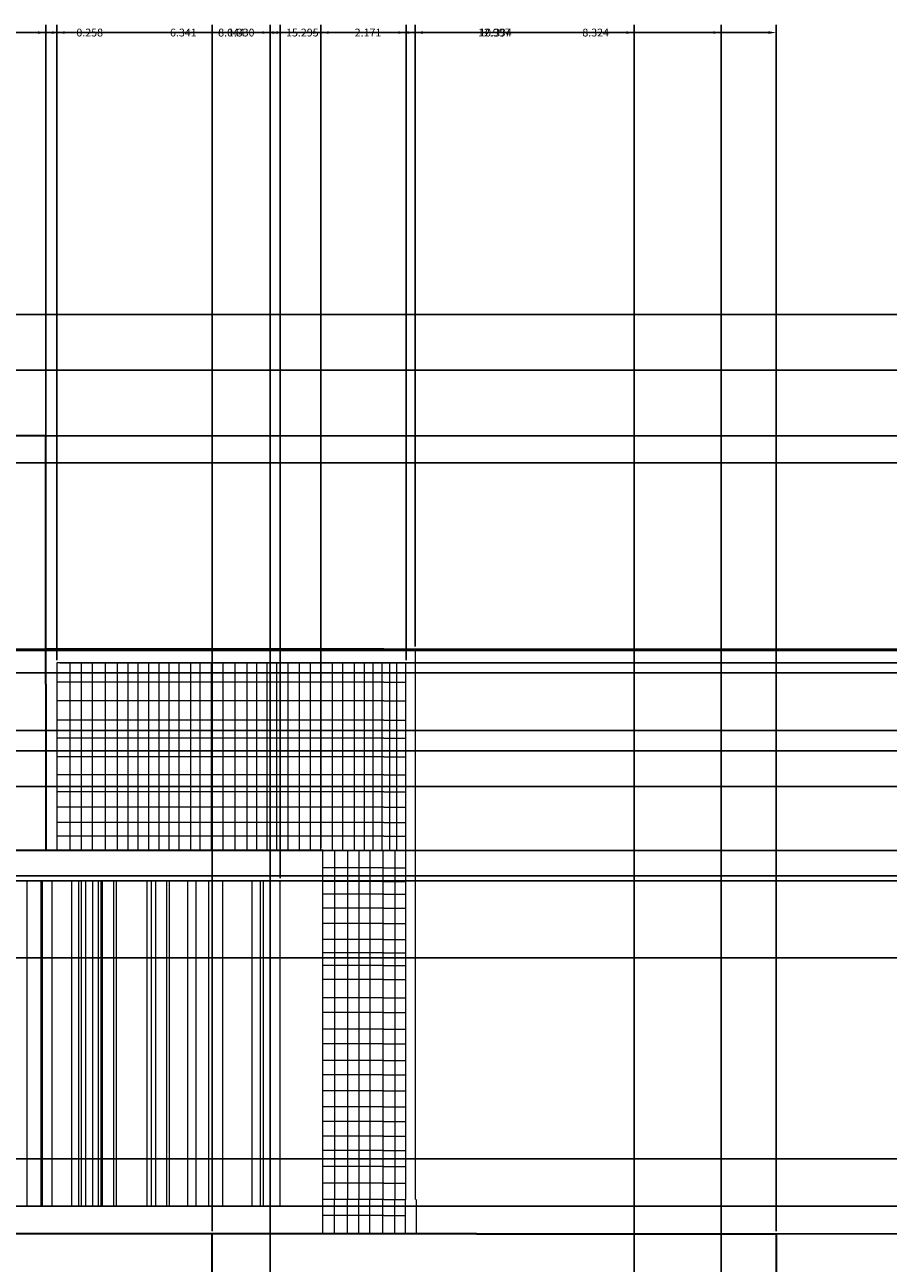
# Model space of a CAD drawing. Units: inches. Extents: x -10 to 130, y -32 to 34.
# Tile 21 of 22: x 90 to 110, y 5 to 34. Entities that reach past the tile are written whole.
import ezdxf

# ---------------------------------------------------------------- set-up
doc = ezdxf.new("R2010")
doc.units = ezdxf.units.IN
doc.header["$MEASUREMENT"] = 0
for name, color, linetype, lineweight in [('A-ANNO-DIMS', 2, 'Continuous', 18), ('A-ELEV', 7, 'Continuous', 35), ('A-GLAZ', 4, 'Continuous', 18)]:
    doc.layers.add(name, color=color, linetype=linetype, lineweight=lineweight)
doc.styles.get("Standard").update_dxf_attribs({"font": 'arial.ttf'})
doc.dimstyles.get("Standard").update_dxf_attribs({"dimtxt": 0.18, "dimasz": 0.18, "dimexe": 0.18, "dimexo": 0.0625, "dimgap": 0.09, "dimtad": 0, "dimtih": 1, "dimtoh": 1, "dimdec": 4, "dimzin": 0, "dimdsep": 46, "dimtxsty": 'Standard', "dimcen": 0.09, "dimadec": 0, "dimazin": 0, "dimtfac": 1, "dimtdec": 4, "dimtofl": 0, "dimtmove": 0, "dimatfit": 3, "dimfxl": 1, "dimtolj": 1, "dimtzin": 0, "dimarcsym": 0})

# ---------------------------------------------------------------- blocks, each defined once
blk = doc.blocks.new('*D2')
at = {"layer": 'A-ANNO-DIMS', "color": 0, "lineweight": -2, "transparency": 16777216}
for p, q in [((68.738, 27.199), (129.508, 27.199)), ((129.328, 27.019), (129.328, 3.074)), ((129.328, -21.234), (129.328, 2.71)), ((107.996, -21.414), (129.508, -21.414))]:
    blk.add_line(p, q, dxfattribs=at)
at = {"layer": 'A-ANNO-DIMS', "color": 0, "transparency": 16777216}
for points in [[(129.298, 27.019), (129.358, 27.019), (129.328, 27.199)], [(129.298, -21.234), (129.358, -21.234), (129.328, -21.414)]]:
    blk.add_solid(points, dxfattribs=at)
at = {"layer": 'Defpoints', "color": 0, "transparency": 16777216}
for p in [(68.676, 27.199), (129.328, 27.199), (107.933, -21.414)]:
    blk.add_point(p, dxfattribs=at)
at = {"layer": 'A-ANNO-DIMS', "color": 0, "transparency": 16777216, "insert": (129.328, 2.892), "char_height": 0.18, "attachment_point": 5}
blk.add_mtext('\\A1;48.61', dxfattribs=at)
blk = doc.blocks.new('*D10')
at = {"layer": 'A-ANNO-DIMS', "color": 0, "lineweight": -2, "transparency": 16777216}
for p, q in [((94.73, 6.07), (94.73, 33.879)), ((94.91, 33.699), (100.773, 33.699)), ((107.547, 33.699), (101.684, 33.699)), ((107.727, 6.07), (107.727, 33.879))]:
    blk.add_line(p, q, dxfattribs=at)
at = {"layer": 'A-ANNO-DIMS', "color": 0, "transparency": 16777216}
for points in [[(94.91, 33.729), (94.91, 33.669), (94.73, 33.699)], [(107.547, 33.729), (107.547, 33.669), (107.727, 33.699)]]:
    blk.add_solid(points, dxfattribs=at)
at = {"layer": 'Defpoints', "color": 0, "transparency": 16777216}
for p in [(107.727, 33.699), (94.73, 6.007), (107.727, 6.007)]:
    blk.add_point(p, dxfattribs=at)
at = {"layer": 'A-ANNO-DIMS', "color": 0, "transparency": 16777216, "insert": (101.229, 33.699), "char_height": 0.18, "attachment_point": 5}
blk.add_mtext('\\A1;12.997', dxfattribs=at)
blk = doc.blocks.new('*D24')
at = {"layer": 'A-ANNO-DIMS', "color": 0, "lineweight": -2, "transparency": 16777216}
for p, q in [((85.383, 19.52), (85.383, 33.879)), ((85.563, 33.699), (87.744, 33.699)), ((90.712, 33.699), (88.531, 33.699)), ((90.892, 24.464), (90.892, 33.879))]:
    blk.add_line(p, q, dxfattribs=at)
at = {"layer": 'A-ANNO-DIMS', "color": 0, "transparency": 16777216}
for points in [[(85.563, 33.729), (85.563, 33.669), (85.383, 33.699)], [(90.712, 33.729), (90.712, 33.669), (90.892, 33.699)]]:
    blk.add_solid(points, dxfattribs=at)
at = {"layer": 'Defpoints', "color": 0, "transparency": 16777216}
for p in [(90.892, 33.699), (90.892, 24.402), (85.383, 19.458)]:
    blk.add_point(p, dxfattribs=at)
at = {"layer": 'A-ANNO-DIMS', "color": 0, "transparency": 16777216, "insert": (88.138, 33.699), "char_height": 0.18, "attachment_point": 5}
blk.add_mtext('\\A1;5.508', dxfattribs=at)
blk = doc.blocks.new('*D25')
at = {"layer": 'A-ANNO-DIMS', "color": 0, "lineweight": -2, "transparency": 16777216}
for p, q in [((90.892, 24.464), (90.892, 33.879)), ((91.072, 33.699), (93.685, 33.699)), ((97.053, 33.699), (94.439, 33.699)), ((97.233, 14.903), (97.233, 33.879))]:
    blk.add_line(p, q, dxfattribs=at)
at = {"layer": 'A-ANNO-DIMS', "color": 0, "transparency": 16777216}
for points in [[(91.072, 33.729), (91.072, 33.669), (90.892, 33.699)], [(97.053, 33.729), (97.053, 33.669), (97.233, 33.699)]]:
    blk.add_solid(points, dxfattribs=at)
at = {"layer": 'Defpoints', "color": 0, "transparency": 16777216}
for p in [(97.233, 33.699), (90.892, 24.402), (97.233, 14.841)]:
    blk.add_point(p, dxfattribs=at)
at = {"layer": 'A-ANNO-DIMS', "color": 0, "transparency": 16777216, "insert": (94.062, 33.699), "char_height": 0.18, "attachment_point": 5}
blk.add_mtext('\\A1;6.341', dxfattribs=at)
blk = doc.blocks.new('*D26')
at = {"layer": 'A-ANNO-DIMS', "color": 0, "lineweight": -2, "transparency": 16777216}
for p, q in [((97.233, 14.903), (97.233, 33.879)), ((97.413, 33.699), (97.94, 33.699)), ((99.223, 33.699), (98.696, 33.699)), ((99.403, 19.547), (99.403, 33.879))]:
    blk.add_line(p, q, dxfattribs=at)
at = {"layer": 'A-ANNO-DIMS', "color": 0, "transparency": 16777216}
for points in [[(97.413, 33.729), (97.413, 33.669), (97.233, 33.699)], [(99.223, 33.729), (99.223, 33.669), (99.403, 33.699)]]:
    blk.add_solid(points, dxfattribs=at)
at = {"layer": 'Defpoints', "color": 0, "transparency": 16777216}
for p in [(99.403, 33.699), (99.403, 19.485), (97.233, 14.841)]:
    blk.add_point(p, dxfattribs=at)
at = {"layer": 'A-ANNO-DIMS', "color": 0, "transparency": 16777216, "insert": (98.318, 33.699), "char_height": 0.18, "attachment_point": 5}
blk.add_mtext('\\A1;2.171', dxfattribs=at)
blk = doc.blocks.new('*D27')
at = {"layer": 'A-ANNO-DIMS', "color": 0, "lineweight": -2, "transparency": 16777216}
for p, q in [((99.403, 19.547), (99.403, 33.879)), ((99.583, 33.699), (103.172, 33.699)), ((107.547, 33.699), (103.959, 33.699)), ((107.727, 6.07), (107.727, 33.879))]:
    blk.add_line(p, q, dxfattribs=at)
at = {"layer": 'A-ANNO-DIMS', "color": 0, "transparency": 16777216}
for points in [[(99.583, 33.729), (99.583, 33.669), (99.403, 33.699)], [(107.547, 33.729), (107.547, 33.669), (107.727, 33.699)]]:
    blk.add_solid(points, dxfattribs=at)
at = {"layer": 'Defpoints', "color": 0, "transparency": 16777216}
for p in [(107.727, 33.699), (99.403, 19.485), (107.727, 6.007)]:
    blk.add_point(p, dxfattribs=at)
at = {"layer": 'A-ANNO-DIMS', "color": 0, "transparency": 16777216, "insert": (103.565, 33.699), "char_height": 0.18, "attachment_point": 5}
blk.add_mtext('\\A1;8.324', dxfattribs=at)
blk = doc.blocks.new('*D29')
at = {"layer": 'A-ANNO-DIMS', "color": 0, "lineweight": -2, "transparency": 16777216}
for p, q in [((69.045, 14.903), (69.045, 33.879)), ((69.225, 33.699), (82.743, 33.699)), ((97.053, 33.699), (83.534, 33.699)), ((97.233, 14.903), (97.233, 33.879))]:
    blk.add_line(p, q, dxfattribs=at)
at = {"layer": 'A-ANNO-DIMS', "color": 0, "transparency": 16777216}
for points in [[(69.225, 33.729), (69.225, 33.669), (69.045, 33.699)], [(97.053, 33.729), (97.053, 33.669), (97.233, 33.699)]]:
    blk.add_solid(points, dxfattribs=at)
at = {"layer": 'Defpoints', "color": 0, "transparency": 16777216}
for p in [(97.233, 33.699), (69.045, 14.841), (97.233, 14.841)]:
    blk.add_point(p, dxfattribs=at)
at = {"layer": 'A-ANNO-DIMS', "color": 0, "transparency": 16777216, "insert": (83.139, 33.699), "char_height": 0.18, "attachment_point": 5}
blk.add_mtext('\\A1;28.19', dxfattribs=at)
blk = doc.blocks.new('*D66')
at = {"layer": 'A-ANNO-DIMS', "color": 0, "lineweight": -2, "transparency": 16777216}
for p, q in [((89.158, -16.844), (89.158, 33.879)), ((89.338, 33.699), (96.35, 33.699)), ((104.273, 33.699), (97.261, 33.699)), ((104.453, -13.219), (104.453, 33.879))]:
    blk.add_line(p, q, dxfattribs=at)
at = {"layer": 'A-ANNO-DIMS', "color": 0, "transparency": 16777216}
for points in [[(89.338, 33.729), (89.338, 33.669), (89.158, 33.699)], [(104.273, 33.729), (104.273, 33.669), (104.453, 33.699)]]:
    blk.add_solid(points, dxfattribs=at)
at = {"layer": 'Defpoints', "color": 0, "transparency": 16777216}
for p in [(104.453, 33.699), (104.453, -13.282), (89.158, -16.906)]:
    blk.add_point(p, dxfattribs=at)
at = {"layer": 'A-ANNO-DIMS', "color": 0, "transparency": 16777216, "insert": (96.805, 33.699), "char_height": 0.18, "attachment_point": 5}
blk.add_mtext('\\A1;15.295', dxfattribs=at)
blk = doc.blocks.new('*D79')
at = {"layer": 'A-ANNO-DIMS', "color": 0, "lineweight": -2, "transparency": 16777216}
for p, q in [((62.588, 7.736), (129.508, 7.736)), ((129.328, 7.556), (129.328, 5.559)), ((129.328, 3.198), (129.328, 5.195)), ((62.588, 3.018), (129.508, 3.018))]:
    blk.add_line(p, q, dxfattribs=at)
at = {"layer": 'A-ANNO-DIMS', "color": 0, "transparency": 16777216}
for points in [[(129.298, 7.556), (129.358, 7.556), (129.328, 7.736)], [(129.298, 3.198), (129.358, 3.198), (129.328, 3.018)]]:
    blk.add_solid(points, dxfattribs=at)
at = {"layer": 'Defpoints', "color": 0, "transparency": 16777216}
for p in [(62.526, 7.736), (129.328, 7.736), (62.526, 3.018)]:
    blk.add_point(p, dxfattribs=at)
at = {"layer": 'A-ANNO-DIMS', "color": 0, "transparency": 16777216, "insert": (129.328, 5.377), "char_height": 0.18, "attachment_point": 5}
blk.add_mtext('\\A1;4.718', dxfattribs=at)
blk = doc.blocks.new('*D80')
at = {"layer": 'A-ANNO-DIMS', "color": 0, "lineweight": -2, "transparency": 16777216}
for p, q in [((62.588, 12.373), (129.508, 12.373)), ((129.328, 12.193), (129.328, 10.237)), ((129.328, 7.916), (129.328, 9.873)), ((62.588, 7.736), (129.508, 7.736))]:
    blk.add_line(p, q, dxfattribs=at)
at = {"layer": 'A-ANNO-DIMS', "color": 0, "transparency": 16777216}
for points in [[(129.298, 12.193), (129.358, 12.193), (129.328, 12.373)], [(129.298, 7.916), (129.358, 7.916), (129.328, 7.736)]]:
    blk.add_solid(points, dxfattribs=at)
at = {"layer": 'Defpoints', "color": 0, "transparency": 16777216}
for p in [(62.526, 12.373), (129.328, 12.373), (62.526, 7.736)]:
    blk.add_point(p, dxfattribs=at)
at = {"layer": 'A-ANNO-DIMS', "color": 0, "transparency": 16777216, "insert": (129.328, 10.055), "char_height": 0.18, "attachment_point": 5}
blk.add_mtext('\\A1;4.64', dxfattribs=at)
blk = doc.blocks.new('*D81')
at = {"layer": 'A-ANNO-DIMS', "color": 0, "lineweight": -2, "transparency": 16777216}
for p, q in [((62.588, 16.317), (129.508, 16.317)), ((129.328, 16.137), (129.328, 14.527)), ((129.328, 12.553), (129.328, 14.163)), ((62.588, 12.373), (129.508, 12.373))]:
    blk.add_line(p, q, dxfattribs=at)
at = {"layer": 'A-ANNO-DIMS', "color": 0, "transparency": 16777216}
for points in [[(129.298, 16.137), (129.358, 16.137), (129.328, 16.317)], [(129.298, 12.553), (129.358, 12.553), (129.328, 12.373)]]:
    blk.add_solid(points, dxfattribs=at)
at = {"layer": 'Defpoints', "color": 0, "transparency": 16777216}
for p in [(62.526, 16.317), (129.328, 16.317), (62.526, 12.373)]:
    blk.add_point(p, dxfattribs=at)
at = {"layer": 'A-ANNO-DIMS', "color": 0, "transparency": 16777216, "insert": (129.328, 14.345), "char_height": 0.18, "attachment_point": 5}
blk.add_mtext('\\A1;3.94', dxfattribs=at)
blk = doc.blocks.new('*D82')
at = {"layer": 'A-ANNO-DIMS', "color": 0, "lineweight": -2, "transparency": 16777216}
for p, q in [((19.651, 19.485), (129.508, 19.485)), ((129.328, 19.305), (129.328, 18.728)), ((129.328, 17.787), (129.328, 18.364)), ((68.738, 17.607), (129.508, 17.607))]:
    blk.add_line(p, q, dxfattribs=at)
at = {"layer": 'A-ANNO-DIMS', "color": 0, "transparency": 16777216}
for points in [[(129.298, 19.305), (129.358, 19.305), (129.328, 19.485)], [(129.298, 17.787), (129.358, 17.787), (129.328, 17.607)]]:
    blk.add_solid(points, dxfattribs=at)
at = {"layer": 'Defpoints', "color": 0, "transparency": 16777216}
for p in [(19.588, 19.485), (68.676, 17.607), (129.328, 17.607)]:
    blk.add_point(p, dxfattribs=at)
at = {"layer": 'A-ANNO-DIMS', "color": 0, "transparency": 16777216, "insert": (129.328, 18.546), "char_height": 0.18, "attachment_point": 5}
blk.add_mtext('\\A1;1.877', dxfattribs=at)
blk = doc.blocks.new('*D85')
at = {"layer": 'A-ANNO-DIMS', "color": 0, "lineweight": -2, "transparency": 16777216}
for p, q in [((50.097, 27.199), (129.508, 27.199)), ((129.328, 27.019), (129.328, 26.738)), ((129.328, 26.093), (129.328, 26.374)), ((51.432, 25.913), (129.508, 25.913))]:
    blk.add_line(p, q, dxfattribs=at)
at = {"layer": 'A-ANNO-DIMS', "color": 0, "transparency": 16777216}
for points in [[(129.298, 27.019), (129.358, 27.019), (129.328, 27.199)], [(129.298, 26.093), (129.358, 26.093), (129.328, 25.913)]]:
    blk.add_solid(points, dxfattribs=at)
at = {"layer": 'Defpoints', "color": 0, "transparency": 16777216}
for p in [(50.035, 27.199), (129.328, 27.199), (51.37, 25.913)]:
    blk.add_point(p, dxfattribs=at)
at = {"layer": 'A-ANNO-DIMS', "color": 0, "transparency": 16777216, "insert": (129.328, 26.556), "char_height": 0.18, "attachment_point": 5}
blk.add_mtext('\\A1;1.286', dxfattribs=at)
blk = doc.blocks.new('*D108')
at = {"layer": 'A-ANNO-DIMS', "color": 0, "lineweight": -2, "transparency": 16777216}
for p, q in [((129.328, 14.841), (129.328, 15.021)), ((129.328, 15.021), (129.508, 15.021)), ((50.009, 14.841), (129.508, 14.841)), ((129.328, 14.436), (129.328, 14.661)), ((49.025, 14.256), (129.508, 14.256))]:
    blk.add_line(p, q, dxfattribs=at)
at = {"layer": 'A-ANNO-DIMS', "color": 0, "transparency": 16777216}
for points in [[(129.298, 14.661), (129.358, 14.661), (129.328, 14.841)], [(129.298, 14.436), (129.358, 14.436), (129.328, 14.256)]]:
    blk.add_solid(points, dxfattribs=at)
at = {"layer": 'Defpoints', "color": 0, "transparency": 16777216}
for p in [(49.946, 14.841), (129.328, 14.841), (48.963, 14.256)]:
    blk.add_point(p, dxfattribs=at)
at = {"layer": 'A-ANNO-DIMS', "color": 0, "transparency": 16777216, "insert": (129.902, 15.021), "char_height": 0.18, "attachment_point": 5}
blk.add_mtext('\\A1;0.585', dxfattribs=at)
blk = doc.blocks.new('*D137')
at = {"layer": 'A-ANNO-DIMS', "color": 0, "lineweight": -2, "transparency": 16777216}
for p, q in [((69.995, 14.206), (69.995, 33.879)), ((70.175, 33.699), (82.678, 33.699)), ((96.113, 33.699), (83.609, 33.699)), ((96.293, 14.206), (96.293, 33.879))]:
    blk.add_line(p, q, dxfattribs=at)
at = {"layer": 'A-ANNO-DIMS', "color": 0, "transparency": 16777216}
for points in [[(70.175, 33.729), (70.175, 33.669), (69.995, 33.699)], [(96.113, 33.729), (96.113, 33.669), (96.293, 33.699)]]:
    blk.add_solid(points, dxfattribs=at)
at = {"layer": 'Defpoints', "color": 0, "transparency": 16777216}
for p in [(96.293, 33.699), (69.995, 14.144), (96.293, 14.144)]:
    blk.add_point(p, dxfattribs=at)
at = {"layer": 'A-ANNO-DIMS', "color": 0, "transparency": 16777216, "insert": (83.144, 33.699), "char_height": 0.18, "attachment_point": 5}
blk.add_mtext('\\A1;26.298', dxfattribs=at)
blk = doc.blocks.new('*D138')
at = {"layer": 'A-ANNO-DIMS', "color": 0, "lineweight": -2, "transparency": 16777216}
for p, q in [((129.328, 14.841), (129.328, 15.021)), ((129.328, 15.021), (129.508, 15.021)), ((69.112, 14.841), (129.508, 14.841)), ((129.328, 14.324), (129.328, 14.661)), ((70.057, 14.144), (129.508, 14.144))]:
    blk.add_line(p, q, dxfattribs=at)
at = {"layer": 'A-ANNO-DIMS', "color": 0, "transparency": 16777216}
for points in [[(129.298, 14.661), (129.358, 14.661), (129.328, 14.841)], [(129.298, 14.324), (129.358, 14.324), (129.328, 14.144)]]:
    blk.add_solid(points, dxfattribs=at)
at = {"layer": 'Defpoints', "color": 0, "transparency": 16777216}
for p in [(69.05, 14.841), (129.328, 14.841), (69.995, 14.144)]:
    blk.add_point(p, dxfattribs=at)
at = {"layer": 'A-ANNO-DIMS', "color": 0, "transparency": 16777216, "insert": (129.901, 15.021), "char_height": 0.18, "attachment_point": 5}
blk.add_mtext('\\A1;0.697', dxfattribs=at)
blk = doc.blocks.new('*D139')
at = {"layer": 'A-ANNO-DIMS', "color": 0, "lineweight": -2, "transparency": 16777216}
for p, q in [((70.057, 6.643), (129.508, 6.643)), ((129.328, 6.463), (129.328, 6.187)), ((69.108, 6.007), (129.508, 6.007)), ((129.328, 6.007), (129.328, 5.827)), ((129.328, 5.827), (129.148, 5.827))]:
    blk.add_line(p, q, dxfattribs=at)
at = {"layer": 'A-ANNO-DIMS', "color": 0, "transparency": 16777216}
for points in [[(129.298, 6.463), (129.358, 6.463), (129.328, 6.643)], [(129.298, 6.187), (129.358, 6.187), (129.328, 6.007)]]:
    blk.add_solid(points, dxfattribs=at)
at = {"layer": 'Defpoints', "color": 0, "transparency": 16777216}
for p in [(69.995, 6.643), (69.045, 6.007), (129.328, 6.007)]:
    blk.add_point(p, dxfattribs=at)
at = {"layer": 'A-ANNO-DIMS', "color": 0, "transparency": 16777216, "insert": (128.754, 5.827), "char_height": 0.18, "attachment_point": 5}
blk.add_mtext('\\A1;0.636', dxfattribs=at)
blk = doc.blocks.new('*D140')
at = {"layer": 'A-ANNO-DIMS', "color": 0, "lineweight": -2, "transparency": 16777216}
for p, q in [((90.712, 33.699), (90.532, 33.699)), ((90.892, 19.547), (90.892, 33.879)), ((91.15, 19.232), (91.15, 33.879)), ((91.33, 33.699), (91.51, 33.699))]:
    blk.add_line(p, q, dxfattribs=at)
at = {"layer": 'A-ANNO-DIMS', "color": 0, "transparency": 16777216}
for points in [[(90.712, 33.729), (90.712, 33.669), (90.892, 33.699)], [(91.33, 33.729), (91.33, 33.669), (91.15, 33.699)]]:
    blk.add_solid(points, dxfattribs=at)
at = {"layer": 'Defpoints', "color": 0, "transparency": 16777216}
for p in [(91.15, 33.699), (90.892, 19.485), (91.15, 19.17)]:
    blk.add_point(p, dxfattribs=at)
at = {"layer": 'A-ANNO-DIMS', "color": 0, "transparency": 16777216, "insert": (91.904, 33.699), "char_height": 0.18, "attachment_point": 5}
blk.add_mtext('\\A1;0.258', dxfattribs=at)
blk = doc.blocks.new('*D141')
at = {"layer": 'A-ANNO-DIMS', "color": 0, "lineweight": -2, "transparency": 16777216}
for p, q in [((91.15, 19.232), (91.15, 33.879)), ((91.33, 33.699), (94.778, 33.699)), ((99.014, 33.699), (95.565, 33.699)), ((99.194, 19.232), (99.194, 33.879))]:
    blk.add_line(p, q, dxfattribs=at)
at = {"layer": 'A-ANNO-DIMS', "color": 0, "transparency": 16777216}
for points in [[(91.33, 33.729), (91.33, 33.669), (91.15, 33.699)], [(99.014, 33.729), (99.014, 33.669), (99.194, 33.699)]]:
    blk.add_solid(points, dxfattribs=at)
at = {"layer": 'Defpoints', "color": 0, "transparency": 16777216}
for p in [(99.194, 33.699), (91.15, 19.17), (99.194, 19.17)]:
    blk.add_point(p, dxfattribs=at)
at = {"layer": 'A-ANNO-DIMS', "color": 0, "transparency": 16777216, "insert": (95.172, 33.699), "char_height": 0.18, "attachment_point": 5}
blk.add_mtext('\\A1;8.044', dxfattribs=at)
blk = doc.blocks.new('*D142')
at = {"layer": 'A-ANNO-DIMS', "color": 0, "lineweight": -2, "transparency": 16777216}
for p, q in [((129.328, 19.665), (129.328, 19.845)), ((129.328, 19.845), (129.508, 19.845)), ((90.954, 19.485), (129.508, 19.485)), ((91.212, 19.17), (129.508, 19.17)), ((129.328, 18.99), (129.328, 18.81))]:
    blk.add_line(p, q, dxfattribs=at)
at = {"layer": 'A-ANNO-DIMS', "color": 0, "transparency": 16777216}
for points in [[(129.298, 19.665), (129.358, 19.665), (129.328, 19.485)], [(129.298, 18.99), (129.358, 18.99), (129.328, 19.17)]]:
    blk.add_solid(points, dxfattribs=at)
at = {"layer": 'Defpoints', "color": 0, "transparency": 16777216}
for p in [(90.892, 19.485), (129.328, 19.485), (91.15, 19.17)]:
    blk.add_point(p, dxfattribs=at)
at = {"layer": 'A-ANNO-DIMS', "color": 0, "transparency": 16777216, "insert": (129.902, 19.845), "char_height": 0.18, "attachment_point": 5}
blk.add_mtext('\\A1;0.315', dxfattribs=at)
blk = doc.blocks.new('*D145')
at = {"layer": 'A-ANNO-DIMS', "color": 0, "lineweight": -2, "transparency": 16777216}
for p, q in [((129.328, 24.402), (129.328, 24.582)), ((129.328, 24.582), (129.508, 24.582)), ((82.677, 24.402), (129.508, 24.402)), ((129.328, 23.959), (129.328, 24.222)), ((83.241, 23.779), (129.508, 23.779))]:
    blk.add_line(p, q, dxfattribs=at)
at = {"layer": 'A-ANNO-DIMS', "color": 0, "transparency": 16777216}
for points in [[(129.298, 24.222), (129.358, 24.222), (129.328, 24.402)], [(129.298, 23.959), (129.358, 23.959), (129.328, 23.779)]]:
    blk.add_solid(points, dxfattribs=at)
at = {"layer": 'Defpoints', "color": 0, "transparency": 16777216}
for p in [(82.614, 24.402), (129.328, 24.402), (83.179, 23.779)]:
    blk.add_point(p, dxfattribs=at)
at = {"layer": 'A-ANNO-DIMS', "color": 0, "transparency": 16777216, "insert": (129.901, 24.582), "char_height": 0.18, "attachment_point": 5}
blk.add_mtext('\\A1;0.623', dxfattribs=at)
blk = doc.blocks.new('*D148')
at = {"layer": 'A-ANNO-DIMS', "color": 0, "lineweight": -2, "transparency": 16777216}
for p, q in [((129.327673, 19.637521), (129.327673, 19.817521)), ((79.689531, 19.457521), (129.507673, 19.457521)), ((80.07533, 18.935883), (129.507673, 18.935883)), ((129.327673, 18.755883), (129.327673, 18.575883))]:
    blk.add_line(p, q, dxfattribs=at)
at = {"layer": 'A-ANNO-DIMS', "color": 0, "transparency": 16777216}
for points in [[(129.297673, 19.637521), (129.357673, 19.637521), (129.327673, 19.457521)], [(129.297673, 18.755883), (129.357673, 18.755883), (129.327673, 18.935883)]]:
    blk.add_solid(points, dxfattribs=at)
at = {"layer": 'Defpoints', "color": 0, "transparency": 16777216}
for p in [(79.627031, 19.457521), (129.327673, 19.457521), (80.01283, 18.935883)]:
    blk.add_point(p, dxfattribs=at)
at = {"layer": 'A-ANNO-DIMS', "color": 0, "transparency": 16777216, "insert": (129.327673, 19.196702), "char_height": 0.18, "attachment_point": 5}
blk.add_mtext('\\A1;0.522', dxfattribs=at)
blk = doc.blocks.new('*D150')
at = {"layer": 'A-ANNO-DIMS', "color": 0, "lineweight": -2, "transparency": 16777216}
for p, q in [((129.327673, 17.787359), (129.327673, 17.967359)), ((74.432221, 17.607359), (129.507673, 17.607359)), ((73.944831, 17.142679), (129.507673, 17.142679)), ((129.327673, 16.962679), (129.327673, 16.782679))]:
    blk.add_line(p, q, dxfattribs=at)
at = {"layer": 'A-ANNO-DIMS', "color": 0, "transparency": 16777216}
for points in [[(129.297673, 17.787359), (129.357673, 17.787359), (129.327673, 17.607359)], [(129.297673, 16.962679), (129.357673, 16.962679), (129.327673, 17.142679)]]:
    blk.add_solid(points, dxfattribs=at)
at = {"layer": 'Defpoints', "color": 0, "transparency": 16777216}
for p in [(74.369721, 17.607359), (129.327673, 17.607359), (73.882331, 17.142679)]:
    blk.add_point(p, dxfattribs=at)
at = {"layer": 'A-ANNO-DIMS', "color": 0, "transparency": 16777216, "insert": (129.327673, 17.375019), "char_height": 0.18, "attachment_point": 5}
blk.add_mtext('\\A1;0.465', dxfattribs=at)
blk = doc.blocks.new('*D154')
at = {"layer": 'A-ANNO-DIMS', "color": 0, "lineweight": -2, "transparency": 16777216}
for p, q in [((81.468, 6.007), (129.508, 6.007)), ((129.328, 5.827), (129.328, 3.941)), ((129.328, 1.691), (129.328, 3.577)), ((81.468, 1.511), (129.508, 1.511))]:
    blk.add_line(p, q, dxfattribs=at)
at = {"layer": 'A-ANNO-DIMS', "color": 0, "transparency": 16777216}
for points in [[(129.298, 5.827), (129.358, 5.827), (129.328, 6.007)], [(129.298, 1.691), (129.358, 1.691), (129.328, 1.511)]]:
    blk.add_solid(points, dxfattribs=at)
at = {"layer": 'Defpoints', "color": 0, "transparency": 16777216}
for p in [(81.405, 6.007), (129.328, 6.007), (81.405, 1.511)]:
    blk.add_point(p, dxfattribs=at)
at = {"layer": 'A-ANNO-DIMS', "color": 0, "transparency": 16777216, "insert": (129.328, 3.759), "char_height": 0.18, "attachment_point": 5}
blk.add_mtext('\\A1;4.497', dxfattribs=at)
blk = doc.blocks.new('*D161')
at = {"layer": 'A-ANNO-DIMS', "color": 0, "lineweight": -2, "transparency": 16777216}
for p, q in [((94.793, 6.007), (129.508, 6.007)), ((129.328, 5.827), (129.328, 5.064)), ((129.328, 3.936), (129.328, 4.7)), ((94.793, 3.756), (129.508, 3.756))]:
    blk.add_line(p, q, dxfattribs=at)
at = {"layer": 'A-ANNO-DIMS', "color": 0, "transparency": 16777216}
for points in [[(129.298, 5.827), (129.358, 5.827), (129.328, 6.007)], [(129.298, 3.936), (129.358, 3.936), (129.328, 3.756)]]:
    blk.add_solid(points, dxfattribs=at)
at = {"layer": 'Defpoints', "color": 0, "transparency": 16777216}
for p in [(94.73, 6.007), (94.73, 3.756), (129.328, 3.756)]:
    blk.add_point(p, dxfattribs=at)
at = {"layer": 'A-ANNO-DIMS', "color": 0, "transparency": 16777216, "insert": (129.328, 4.882), "char_height": 0.18, "attachment_point": 5}
blk.add_mtext('\\A1;2.252', dxfattribs=at)
blk = doc.blocks.new('*D163')
at = {"layer": 'A-ANNO-DIMS', "color": 0, "lineweight": -2, "transparency": 16777216}
for p, q in [((94.73, 6.07), (94.73, 33.879)), ((94.91, 33.699), (95.01, 33.699)), ((95.881, 33.699), (95.78, 33.699)), ((96.061, 5.012), (96.061, 33.879))]:
    blk.add_line(p, q, dxfattribs=at)
at = {"layer": 'A-ANNO-DIMS', "color": 0, "transparency": 16777216}
for points in [[(94.91, 33.729), (94.91, 33.669), (94.73, 33.699)], [(95.881, 33.729), (95.881, 33.669), (96.061, 33.699)]]:
    blk.add_solid(points, dxfattribs=at)
at = {"layer": 'Defpoints', "color": 0, "transparency": 16777216}
for p in [(96.061, 33.699), (94.73, 6.007), (96.061, 4.95)]:
    blk.add_point(p, dxfattribs=at)
at = {"layer": 'A-ANNO-DIMS', "color": 0, "transparency": 16777216, "insert": (95.395, 33.699), "char_height": 0.18, "attachment_point": 5}
blk.add_mtext('\\A1;1.330', dxfattribs=at)
blk = doc.blocks.new('*D164')
at = {"layer": 'A-ANNO-DIMS', "color": 0, "lineweight": -2, "transparency": 16777216}
for p, q in [((96.061, 5.012), (96.061, 33.879)), ((96.241, 33.699), (100.803, 33.699)), ((106.274, 33.699), (101.712, 33.699)), ((106.454, 5.012), (106.454, 33.879))]:
    blk.add_line(p, q, dxfattribs=at)
at = {"layer": 'A-ANNO-DIMS', "color": 0, "transparency": 16777216}
for points in [[(96.241, 33.729), (96.241, 33.669), (96.061, 33.699)], [(106.274, 33.729), (106.274, 33.669), (106.454, 33.699)]]:
    blk.add_solid(points, dxfattribs=at)
at = {"layer": 'Defpoints', "color": 0, "transparency": 16777216}
for p in [(106.454, 33.699), (96.061, 4.95), (106.454, 4.95)]:
    blk.add_point(p, dxfattribs=at)
at = {"layer": 'A-ANNO-DIMS', "color": 0, "transparency": 16777216, "insert": (101.257, 33.699), "char_height": 0.18, "attachment_point": 5}
blk.add_mtext('\\A1;10.394', dxfattribs=at)
blk = doc.blocks.new('*D165')
at = {"layer": 'A-ANNO-DIMS', "color": 0, "lineweight": -2, "transparency": 16777216}
for p, q in [((94.793, 6.007), (129.508, 6.007)), ((129.328, 5.827), (129.328, 5.66)), ((129.328, 5.13), (129.328, 5.297)), ((96.123, 4.95), (129.508, 4.95))]:
    blk.add_line(p, q, dxfattribs=at)
at = {"layer": 'A-ANNO-DIMS', "color": 0, "transparency": 16777216}
for points in [[(129.298, 5.827), (129.358, 5.827), (129.328, 6.007)], [(129.298, 5.13), (129.358, 5.13), (129.328, 4.95)]]:
    blk.add_solid(points, dxfattribs=at)
at = {"layer": 'Defpoints', "color": 0, "transparency": 16777216}
for p in [(94.73, 6.007), (129.328, 6.007), (96.061, 4.95)]:
    blk.add_point(p, dxfattribs=at)
at = {"layer": 'A-ANNO-DIMS', "color": 0, "transparency": 16777216, "insert": (129.328, 5.478), "char_height": 0.18, "attachment_point": 5}
blk.add_mtext('\\A1;1.058', dxfattribs=at)

msp = doc.modelspace()

# ---------------------------------------------------------------- linework, layer by layer
at = {"layer": 'A-ELEV'}
for p, q in [((90.8917, 24.4019), (82.6141, 24.4019)), ((90.8917, 18.6807), (90.8917, 24.4019)), ((98.6791, 19.4845), (90.8917, 19.4845)), ((90.8917, 18.6807), (90.8917, 14.8409)), ((97.276, 14.8409), (69.0452, 14.8409)), ((98.6791, 6.0074), (69.0452, 6.0074)), ((94.7302, -6.2218), (94.7302, 6.0074)), ((100.8166, 6.0074), (97.276, 6.0074)), ((100.8166, 6.0074), (101.5409, 6.0074)), ((101.5409, 6.0074), (107.7269, 6.0074)), ((107.7269, 6.0074), (107.7269, -6.2218))]:
    msp.add_line(p, q, dxfattribs=at)
at = {"layer": 'A-GLAZ'}
for p, q in [((98.6791, 19.4845), (99.4034, 19.4845)), ((99.4034, 19.4845), (99.4034, 18.6807)), ((98.6791, 19.1697), (91.1497, 19.1697)), ((91.1497, 19.1697), (91.1497, 18.6807)), ((91.4435, 19.1697), (91.4435, 18.6807)), ((91.71, 19.1697), (91.71, 18.6807)), ((91.9628, 19.1697), (91.9628, 18.6807)), ((92.2634, 19.1697), (92.2634, 18.6807)), ((92.5367, 19.1697), (92.5367, 18.6807)), ((92.7827, 19.1697), (92.7827, 18.6807)), ((93.0174, 14.8409), (93.0174, 19.1697)), ((93.2654, 14.8409), (93.2654, 19.1697)), ((93.5021, 14.8409), (93.5021, 19.1697)), ((93.7387, 14.8409), (93.7387, 19.1697)), ((93.9641, 14.8409), (93.9641, 19.1697)), ((94.2346, 14.8409), (94.2346, 19.1697)), ((94.4488, 14.8409), (94.4488, 19.1697)), ((94.708, 14.8409), (94.708, 19.1697)), ((94.9785, 14.8409), (94.9785, 19.1697)), ((95.2602, 14.8409), (95.2602, 19.1697)), ((95.5307, 14.8409), (95.5307, 19.1697)), ((95.7561, 14.8409), (95.7561, 19.1697)), ((95.9928, 14.8409), (95.9928, 19.1697)), ((96.2182, 14.8409), (96.2182, 19.1697)), ((96.4774, 14.8409), (96.4774, 19.1697)), ((96.7366, 14.8409), (96.7366, 19.1697)), ((96.9959, 14.8409), (96.9959, 19.1697)), ((97.2325, 14.8409), (97.2325, 19.1697)), ((97.503, 14.8409), (97.503, 19.1697)), ((97.7397, 14.8409), (97.7397, 19.1697)), ((98.0102, 14.8409), (98.0102, 19.1697)), ((98.2356, 14.8409), (98.2356, 19.1697)), ((98.4385, 14.8409), (98.4385, 19.1697)), ((98.6413, 14.8409), (98.6413, 19.1697)), ((98.6791, 19.1697), (99.1936, 19.1697)), ((98.8216, 14.8409), (98.8216, 19.1697)), ((98.9794, 14.8409), (98.9794, 19.1697)), ((99.1936, 14.8409), (99.1936, 19.1697)), ((98.6791, 18.7245), (91.1497, 18.7245)), ((91.1497, 18.6807), (91.1497, 15.1746)), ((91.4435, 18.6807), (91.4435, 15.1746)), ((91.71, 18.6807), (91.71, 15.1746)), ((91.9628, 18.6807), (91.9628, 15.1746)), ((92.2634, 18.6807), (92.2634, 15.1746)), ((92.5367, 18.6807), (92.5367, 15.1746)), ((92.7827, 18.6807), (92.7827, 15.1746)), ((98.6791, 18.7245), (99.1936, 18.7245)), ((99.4034, 18.6807), (99.4034, 6.7976)), ((98.6791, 18.2941), (91.1497, 18.2941)), ((98.6791, 18.2941), (99.1936, 18.2941)), ((98.6791, 17.8489), (91.1497, 17.8489)), ((98.6791, 17.8489), (99.1936, 17.8489)), ((98.6791, 17.4334), (91.1497, 17.4334)), ((98.6791, 17.4334), (99.1936, 17.4334)), ((98.6791, 17.0031), (91.1497, 17.0031)), ((98.6791, 17.0031), (99.1936, 17.0031)), ((98.6791, 16.5876), (91.1497, 16.5876)), ((98.6791, 16.5876), (99.1936, 16.5876)), ((98.6791, 16.1986), (91.1497, 16.1986)), ((98.6791, 16.1986), (99.1936, 16.1986)), ((98.6791, 15.8424), (91.1497, 15.8424)), ((98.6791, 15.8424), (99.1936, 15.8424)), ((98.6791, 15.4863), (91.1497, 15.4863)), ((98.6791, 15.4863), (99.1936, 15.4863)), ((98.6791, 15.1746), (91.1497, 15.1746)), ((91.1497, 15.1746), (91.1497, 14.8409)), ((91.4435, 15.1746), (91.4435, 14.8409)), ((91.71, 15.1746), (91.71, 14.8409)), ((91.9628, 15.1746), (91.9628, 14.8409)), ((92.2634, 15.1746), (92.2634, 14.8409)), ((92.5367, 15.1746), (92.5367, 14.8409)), ((92.7827, 15.1746), (92.7827, 14.8409)), ((98.6791, 15.1746), (99.1936, 15.1746)), ((97.276, 6.0074), (97.276, 14.8409)), ((97.276, 14.8409), (99.1936, 14.8409)), ((97.549, 14.8409), (97.549, 6.7976)), ((97.8428, 14.8409), (97.8428, 6.7976)), ((98.1093, 14.8409), (98.1093, 6.7976)), ((98.3621, 14.8409), (98.3621, 6.7976)), ((98.6627, 14.8409), (98.6627, 6.7976)), ((98.936, 14.8409), (98.936, 6.7976)), ((99.182, 14.8409), (99.182, 6.7976)), ((98.6791, 14.4405), (97.276, 14.4405)), ((98.6791, 14.4405), (99.182, 14.4405)), ((96.2927, 14.144), (69.9946, 14.144)), ((90.4595, 6.6433), (90.4595, 14.144)), ((90.7817, 6.6433), (90.7817, 14.144)), ((90.814, 6.6433), (90.814, 14.144)), ((91.0396, 6.6433), (91.0396, 14.144)), ((91.4908, 6.6433), (91.4908, 14.144)), ((91.6519, 6.6433), (91.6519, 14.144)), ((91.7163, 6.6433), (91.7163, 14.144)), ((91.813, 6.6433), (91.813, 14.144)), ((91.9742, 6.6433), (91.9742, 14.144)), ((91.9742, 6.6433), (91.9742, 14.144)), ((92.1031, 6.6433), (92.1031, 14.144)), ((92.1675, 6.6433), (92.1675, 14.144)), ((92.1998, 6.6433), (92.1998, 14.144)), ((92.4576, 6.6433), (92.4576, 14.144)), ((92.5221, 6.6433), (92.5221, 14.144)), ((93.2311, 6.6433), (93.2311, 14.144)), ((93.2311, 6.6433), (93.2311, 14.144)), ((93.3278, 6.6433), (93.3278, 14.144)), ((93.3278, 6.6433), (93.3278, 14.144)), ((93.4244, 6.6433), (93.4244, 14.144)), ((93.6823, 6.6433), (93.6823, 14.144)), ((93.7467, 6.6433), (93.7467, 14.144)), ((94.1657, 6.6433), (94.1657, 14.144)), ((94.3591, 6.6433), (94.3591, 14.144)), ((94.6491, 6.6433), (94.6491, 14.144)), ((94.9714, 6.6433), (94.9714, 14.144)), ((95.6482, 6.6433), (95.6482, 14.144)), ((95.8415, 6.6433), (95.8415, 14.144)), ((95.906, 6.6433), (95.906, 14.144)), ((96.2927, 6.6433), (96.2927, 14.144)), ((98.6791, 14.1324), (97.276, 14.1324)), ((98.6791, 14.1324), (99.182, 14.1324)), ((98.6791, 13.8397), (97.276, 13.8397)), ((98.6791, 13.8397), (99.182, 13.8397)), ((98.6791, 13.5162), (97.276, 13.5162)), ((98.6791, 13.5162), (99.182, 13.5162)), ((98.6791, 13.1619), (97.276, 13.1619)), ((98.6791, 13.1619), (99.182, 13.1619)), ((98.6791, 12.7922), (97.276, 12.7922)), ((98.6791, 12.7922), (99.182, 12.7922)), ((98.6791, 12.4841), (97.276, 12.4841)), ((98.6791, 12.4841), (99.182, 12.4841)), ((98.6791, 12.1914), (97.276, 12.1914)), ((98.6791, 12.1914), (99.182, 12.1914)), ((98.6791, 11.8679), (97.276, 11.8679)), ((98.6791, 11.8679), (99.182, 11.8679)), ((98.6791, 11.4484), (97.276, 11.4484)), ((98.6791, 11.4484), (99.182, 11.4484)), ((98.6791, 11.1095), (97.276, 11.1095)), ((98.6791, 11.1095), (99.182, 11.1095)), ((98.6791, 10.7244), (97.276, 10.7244)), ((98.6791, 10.7244), (99.182, 10.7244)), ((98.6791, 10.3855), (97.276, 10.3855)), ((98.6791, 10.3855), (99.182, 10.3855)), ((98.6791, 10.0004), (97.276, 10.0004)), ((98.6791, 10.0004), (99.182, 10.0004)), ((98.6791, 9.6726), (97.276, 9.6726)), ((98.6791, 9.6726), (99.182, 9.6726)), ((98.6791, 9.3028), (97.276, 9.3028)), ((98.6791, 9.3028), (99.182, 9.3028)), ((98.6791, 8.9331), (97.276, 8.9331)), ((98.6791, 8.9331), (99.182, 8.9331)), ((98.6791, 8.5942), (97.276, 8.5942)), ((98.6791, 8.5942), (99.182, 8.5942)), ((98.6791, 8.2553), (97.276, 8.2553)), ((98.6791, 8.2553), (99.182, 8.2553)), ((98.6791, 7.9319), (97.276, 7.9319)), ((98.6791, 7.9319), (99.182, 7.9319)), ((98.6791, 7.5621), (97.276, 7.5621)), ((98.6791, 7.5621), (99.182, 7.5621)), ((98.6791, 7.1718), (97.276, 7.1718)), ((98.6791, 7.1718), (99.182, 7.1718)), ((96.2927, 6.6433), (69.9946, 6.6433)), ((98.6791, 6.8021), (97.276, 6.8021)), ((97.549, 6.0074), (97.549, 6.7976)), ((97.8428, 6.0074), (97.8428, 6.7976)), ((98.1093, 6.0074), (98.1093, 6.7976)), ((98.3621, 6.0074), (98.3621, 6.7976)), ((98.6627, 6.0074), (98.6627, 6.7976)), ((98.6791, 6.8021), (99.182, 6.8021)), ((98.936, 6.0074), (98.936, 6.7976)), ((99.182, 6.0074), (99.182, 6.7976)), ((99.4258, 6.7976), (99.4258, 6.0074)), ((98.6791, 6.4324), (97.276, 6.4324)), ((98.6791, 6.4324), (99.182, 6.4324)), ((99.4258, 6.0074), (98.7016, 6.0074))]:
    msp.add_line(p, q, dxfattribs=at)

# ---------------------------------------------------------------- dimensions: what is measured, and where the dimension line sits
at = {"layer": 'A-ANNO-DIMS'}
for base, p1, p2, override, picture, middle in [((97.2325, 33.6987), (69.0452, 14.8409), (97.2325, 14.8409), {"dimdec": 2, "dimlfac": 1, "dimrnd": 0, "dimzin": 0, "dimdsep": 46, "dimlunit": 2}, '*D29', (83.1389, 33.6987)), ((96.2927, 33.6987), (69.9946, 14.144), (96.2927, 14.144), {"dimdec": 3, "dimlfac": 1, "dimrnd": 0, "dimzin": 0, "dimdsep": 46, "dimlunit": 2}, '*D137', (83.1437, 33.6987)), ((90.8917, 33.6987), (85.3833, 19.4575), (90.8917, 24.4019), {"dimdec": 3, "dimlfac": 1, "dimrnd": 0, "dimzin": 0, "dimdsep": 46, "dimlunit": 2}, '*D24', (88.1375, 33.6987)), ((104.4531, 33.6987), (89.1578, -16.9063), (104.4531, -13.2819), {"dimdec": 3, "dimlfac": 1, "dimrnd": 0, "dimzin": 0, "dimdsep": 46, "dimlunit": 2}, '*D66', (96.8055, 33.6987)), ((91.1497, 33.6987), (90.8917, 19.4845), (91.1497, 19.1697), {"dimdec": 3, "dimlfac": 1, "dimrnd": 0, "dimzin": 0, "dimdsep": 46, "dimlunit": 2}, '*D140', (91.9036, 33.6987)), ((97.2325, 33.6987), (90.8917, 24.4019), (97.2325, 14.8409), {"dimdec": 3, "dimlfac": 1, "dimrnd": 0, "dimzin": 0, "dimdsep": 46, "dimlunit": 2}, '*D25', (94.0621, 33.6987)), ((99.1936, 33.6987), (91.1497, 19.1697), (99.1936, 19.1697), {"dimdec": 3, "dimlfac": 1, "dimrnd": 0, "dimzin": 0, "dimdsep": 46, "dimlunit": 2}, '*D141', (95.1716, 33.6987)), ((107.7269, 33.6987), (94.7302, 6.0074), (107.7269, 6.0074), {"dimdec": 3, "dimlfac": 1, "dimrnd": 0, "dimzin": 0, "dimdsep": 46, "dimlunit": 2}, '*D10', (101.2286, 33.6987)), ((96.0606, 33.6987), (94.7302, 6.0074), (96.0606, 4.9495), {"dimdec": 3, "dimlfac": 1, "dimrnd": 0, "dimzin": 0, "dimdsep": 46, "dimlunit": 2}, '*D163', (95.3954, 33.6987)), ((106.4542, 33.6987), (96.0606, 4.9495), (106.4542, 4.9495), {"dimdec": 3, "dimlfac": 1, "dimrnd": 0, "dimzin": 0, "dimdsep": 46, "dimlunit": 2}, '*D164', (101.2574, 33.6987)), ((99.4034, 33.6987), (97.2325, 14.8409), (99.4034, 19.4845), {"dimdec": 3, "dimlfac": 1, "dimrnd": 0, "dimzin": 0, "dimdsep": 46, "dimlunit": 2}, '*D26', (98.318, 33.6987)), ((107.72689, 33.69866), (99.40337, 19.48451), (107.72689, 6.00744), {"dimdec": 3, "dimlfac": 1, "dimrnd": 0, "dimzin": 0, "dimdsep": 46, "dimlunit": 2}, '*D27', (103.56513, 33.69866))]:
    dim = msp.add_linear_dim(base=base, p1=p1, p2=p2, dimstyle='Standard', override=override, dxfattribs=at)
    dim.commit()
    dim.dimension.update_dxf_attribs({"geometry": picture, "text_midpoint": middle})
for base, p1, p2, override, picture, middle in [((129.3277, 27.1987), (51.3699, 25.9127), (50.0347, 27.1987), {"dimdec": 3, "dimlfac": 1, "dimrnd": 0, "dimzin": 0, "dimdsep": 46, "dimlunit": 2}, '*D85', (129.3277, 26.5557)), ((129.3277, 27.1987), (107.9333, -21.4145), (68.6759, 27.1987), {"dimdec": 2, "dimlfac": 1, "dimrnd": 0, "dimzin": 0, "dimdsep": 46, "dimlunit": 2}, '*D2', (129.3277, 2.8921)), ((129.3277, 24.4019), (83.1789, 23.7785), (82.6141, 24.4019), {"dimdec": 3, "dimlfac": 1, "dimrnd": 0, "dimzin": 0, "dimdsep": 46, "dimlunit": 2}, '*D145', (129.9014, 24.5819)), ((129.3277, 19.4575), (80.0128, 18.9359), (79.627, 19.4575), {"dimdec": 3, "dimlfac": 1, "dimrnd": 0, "dimzin": 0, "dimdsep": 46, "dimlunit": 2}, '*D148', (129.3277, 19.1967)), ((129.3277, 19.4845), (91.1497, 19.1697), (90.8917, 19.4845), {"dimdec": 3, "dimlfac": 1, "dimrnd": 0, "dimzin": 0, "dimdsep": 46, "dimlunit": 2}, '*D142', (129.9021, 19.8445)), ((129.3277, 17.6074), (19.5881, 19.4845), (68.6759, 17.6074), {"dimdec": 3, "dimlfac": 1, "dimrnd": 0, "dimzin": 0, "dimdsep": 46, "dimlunit": 2}, '*D82', (129.3277, 18.5459)), ((129.3277, 17.6074), (73.8823, 17.1427), (74.3697, 17.6074), {"dimdec": 3, "dimlfac": 1, "dimrnd": 0, "dimzin": 0, "dimdsep": 46, "dimlunit": 2}, '*D150', (129.3277, 17.375)), ((129.3277, 16.3174), (62.5256, 12.3729), (62.5256, 16.3174), {"dimdec": 2, "dimlfac": 1, "dimrnd": 0, "dimzin": 0, "dimdsep": 46, "dimlunit": 2}, '*D81', (129.3277, 14.3452)), ((129.3277, 14.8409), (48.963, 14.2556), (49.9462, 14.8409), {"dimdec": 3, "dimlfac": 1, "dimrnd": 0, "dimzin": 0, "dimdsep": 46, "dimlunit": 2}, '*D108', (129.9021, 15.0209)), ((129.3277, 14.8409), (69.9946, 14.144), (69.0498, 14.8409), {"dimdec": 3, "dimlfac": 1, "dimrnd": 0, "dimzin": 0, "dimdsep": 46, "dimlunit": 2}, '*D138', (129.9014, 15.0209)), ((129.3277, 12.3729), (62.5256, 7.7364), (62.5256, 12.3729), {"dimdec": 2, "dimlfac": 1, "dimrnd": 0, "dimzin": 0, "dimdsep": 46, "dimlunit": 2}, '*D80', (129.3277, 10.0547)), ((129.3277, 7.7364), (62.5256, 3.0181), (62.5256, 7.7364), {"dimdec": 3, "dimlfac": 1, "dimrnd": 0, "dimzin": 0, "dimdsep": 46, "dimlunit": 2}, '*D79', (129.3277, 5.3773)), ((129.3277, 6.0074), (69.9946, 6.6433), (69.0452, 6.0074), {"dimdec": 3, "dimlfac": 1, "dimrnd": 0, "dimzin": 0, "dimdsep": 46, "dimlunit": 2}, '*D139', (128.754, 5.8274)), ((129.3277, 6.0074), (81.4053, 1.5107), (81.4053, 6.0074), {"dimdec": 3, "dimlfac": 1, "dimrnd": 0, "dimzin": 0, "dimdsep": 46, "dimlunit": 2}, '*D154', (129.3277, 3.7591)), ((129.3277, 3.7558), (94.7302, 6.0074), (94.7302, 3.7558), {"dimdec": 3, "dimlfac": 1, "dimrnd": 0, "dimzin": 0, "dimdsep": 46, "dimlunit": 2}, '*D161', (129.3277, 4.8816)), ((129.3277, 6.0074), (96.0606, 4.9495), (94.7302, 6.0074), {"dimdec": 3, "dimlfac": 1, "dimrnd": 0, "dimzin": 0, "dimdsep": 46, "dimlunit": 2}, '*D165', (129.3277, 5.4785))]:
    dim = msp.add_linear_dim(base=base, p1=p1, p2=p2, angle=90, dimstyle='Standard', override=override, dxfattribs=at)
    dim.commit()
    dim.dimension.update_dxf_attribs({"geometry": picture, "text_midpoint": middle})

doc.saveas('drawing.dxf')
